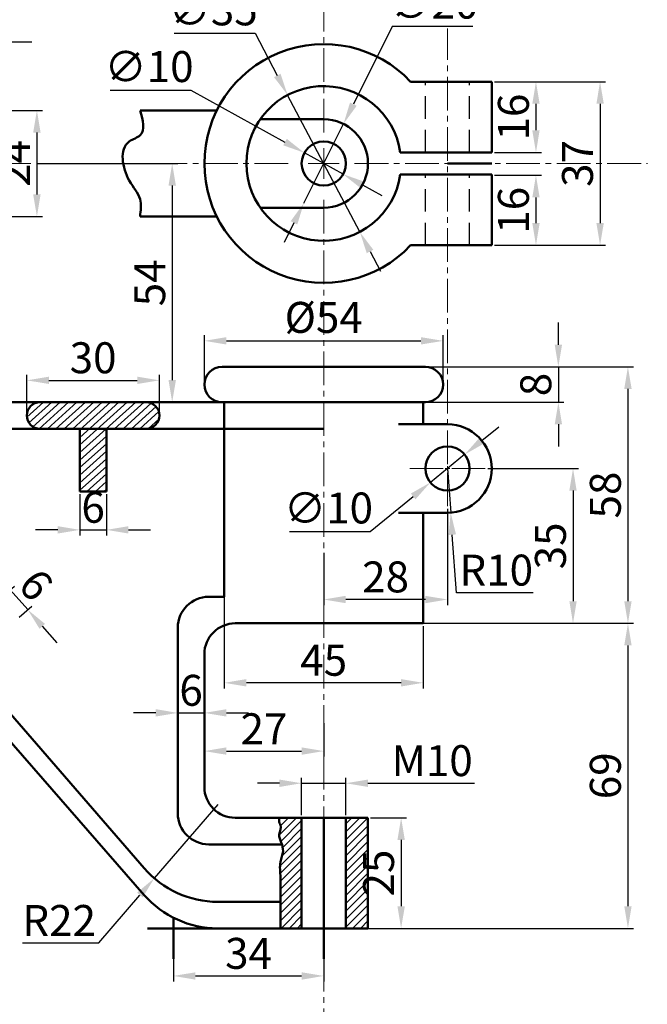
# Model space of a CAD drawing. Units: millimetres. Extents: x 434 to 1535, y -197 to 318.
# Tile 2 of 9: x 579 to 721, y -19 to 204. Entities that reach past the tile are written whole.
import ezdxf

# ---------------------------------------------------------------- set-up
doc = ezdxf.new("R2010")
doc.units = ezdxf.units.MM
doc.header["$LTSCALE"] = 0.4
doc.linetypes.add('CENTER2', pattern=[28.575, 19.05, -3.175, 3.175, -3.175])
doc.linetypes.add('DASHED', pattern=[19.05, 12.7, -6.35])
for name, color, linetype, lineweight in [('M-CNTR', 1, 'CENTER2', 18), ('M-DIMS', 2, 'Continuous', 25), ('M-HATC', 8, 'Continuous', 18), ('M-HIDN', 6, 'DASHED', 25), ('M-OUTL', 7, 'Continuous', 50)]:
    doc.layers.add(name, color=color, linetype=linetype, lineweight=lineweight)
doc.styles.get("Standard").update_dxf_attribs({"font": 'arial.ttf'})
doc.dimstyles.new('ISO-25', dxfattribs={"dimtxt": 7, "dimasz": 5, "dimexe": 1.25, "dimexo": 0.625, "dimtad": 1, "dimtoh": 1, "dimdec": 0, "dimtxsty": 'Standard', "dimcen": 2.5, "dimadec": 0, "dimazin": 0, "dimtfac": 1, "dimtdec": 0, "dimtmove": 0, "dimatfit": 3, "dimfxl": 1, "dimarcsym": 0})

# ---------------------------------------------------------------- blocks, each defined once
blk = doc.blocks.new('*U1')
at = {"layer": 'M-CNTR', "color": 0, "transparency": 16777216}
for p, q in [((0, 7), (0, 38.5)), ((-38.5, 0), (-7, 0)), ((7, 0), (73.2, 0)), ((0, -198.75), (0, -7))]:
    blk.add_line(p, q, dxfattribs=at)
at = {"layer": 'M-CNTR', "color": 0, "linetype": 'Continuous', "transparency": 16777216}
for p, q in [((0, -3.5), (0, 3.5)), ((-3.5, 0), (3.5, 0))]:
    blk.add_line(p, q, dxfattribs=at)
blk = doc.blocks.new('*U2')
at = {"layer": 'M-CNTR', "color": 0, "transparency": 16777216}
for p, q in [((0, 1), (0, 99.51)), ((-8.5, 0), (-1, 0)), ((1, 0), (8.5, 0)), ((0, -8.5), (0, -1))]:
    blk.add_line(p, q, dxfattribs=at)
at = {"layer": 'M-CNTR', "color": 0, "linetype": 'Continuous', "transparency": 16777216}
for p, q in [((-0.5, 0), (0.5, 0)), ((0, -0.5), (0, 0.5))]:
    blk.add_line(p, q, dxfattribs=at)
blk = doc.blocks.new('*U3')
at = {"layer": 'M-CNTR', "color": 0, "transparency": 16777216}
blk.add_line((-45.89, 0), (45.61, 0), dxfattribs=at)
blk = doc.blocks.new('*D12')
at = {"layer": 'Defpoints', "color": 0, "ltscale": 0.4, "transparency": 16777216}
for p in [(571.58, 199.04), (563.58, 188.56), (571.58, 188.56)]:
    blk.add_point(p, dxfattribs=at)
at = {"layer": 'M-DIMS', "color": 0, "lineweight": -2, "ltscale": 0.4, "transparency": 16777216}
for p, q in [((558.58, 199.04), (553.58, 199.04)), ((563.58, 189.19), (563.58, 200.29)), ((563.58, 199.04), (571.58, 199.04)), ((571.58, 189.19), (571.58, 200.29)), ((576.58, 199.04), (581.58, 199.04))]:
    blk.add_line(p, q, dxfattribs=at)
at = {"layer": 'M-DIMS', "color": 0, "ltscale": 0.4, "transparency": 16777216}
for points in [[(558.58, 199.87), (558.58, 198.21), (563.58, 199.04)], [(576.58, 199.87), (576.58, 198.21), (571.58, 199.04)]]:
    blk.add_solid(points, dxfattribs=at)
at = {"layer": 'M-DIMS', "color": 0, "ltscale": 0.4, "transparency": 16777216, "insert": (567.58, 203.24), "char_height": 7, "attachment_point": 5}
blk.add_mtext('8', dxfattribs=at)
blk = doc.blocks.new('*D13')
at = {"layer": 'Defpoints', "color": 0, "ltscale": 0.4, "transparency": 16777216}
for p in [(571.58, 183.56), (571.58, 159.56), (582.71, 159.56)]:
    blk.add_point(p, dxfattribs=at)
at = {"layer": 'M-DIMS', "color": 0, "lineweight": -2, "ltscale": 0.4, "transparency": 16777216}
for p, q in [((572.2, 183.56), (583.96, 183.56)), ((582.71, 178.56), (582.71, 164.56)), ((572.2, 159.56), (583.96, 159.56))]:
    blk.add_line(p, q, dxfattribs=at)
at = {"layer": 'M-DIMS', "color": 0, "ltscale": 0.4, "transparency": 16777216}
for points in [[(581.87, 178.56), (583.54, 178.56), (582.71, 183.56)], [(581.87, 164.56), (583.54, 164.56), (582.71, 159.56)]]:
    blk.add_solid(points, dxfattribs=at)
at = {"layer": 'M-DIMS', "color": 0, "ltscale": 0.4, "transparency": 16777216, "insert": (578.57, 171.56), "char_height": 7, "attachment_point": 5, "rotation": 90}
blk.add_mtext('24', dxfattribs=at)
blk = doc.blocks.new('*D17')
at = {"layer": 'Defpoints', "color": 0, "ltscale": 0.4, "transparency": 16777216}
for p in [(610.41, 122.51), (580.43, 114.31), (610.41, 114.31)]:
    blk.add_point(p, dxfattribs=at)
at = {"layer": 'M-DIMS', "color": 0, "lineweight": -2, "ltscale": 0.4, "transparency": 16777216}
for p, q in [((580.43, 114.93), (580.43, 123.76)), ((585.43, 122.51), (605.41, 122.51)), ((610.41, 114.93), (610.41, 123.76))]:
    blk.add_line(p, q, dxfattribs=at)
at = {"layer": 'M-DIMS', "color": 0, "ltscale": 0.4, "transparency": 16777216}
for points in [[(585.43, 123.34), (585.43, 121.68), (580.43, 122.51)], [(605.41, 123.34), (605.41, 121.68), (610.41, 122.51)]]:
    blk.add_solid(points, dxfattribs=at)
at = {"layer": 'M-DIMS', "color": 0, "ltscale": 0.4, "transparency": 16777216, "insert": (595.42, 126.71), "char_height": 7, "attachment_point": 5}
blk.add_mtext('30', dxfattribs=at)
blk = doc.blocks.new('*D18')
at = {"layer": 'Defpoints', "color": 0, "ltscale": 0.4, "transparency": 16777216}
for p in [(592.42, 97.38), (598.42, 97.38), (598.42, 88.69)]:
    blk.add_point(p, dxfattribs=at)
at = {"layer": 'M-DIMS', "color": 0, "lineweight": -2, "ltscale": 0.4, "transparency": 16777216}
for p, q in [((592.42, 96.75), (592.42, 87.44)), ((598.42, 96.75), (598.42, 87.44)), ((587.42, 88.69), (582.42, 88.69)), ((592.42, 88.69), (598.42, 88.69)), ((603.42, 88.69), (608.42, 88.69))]:
    blk.add_line(p, q, dxfattribs=at)
at = {"layer": 'M-DIMS', "color": 0, "ltscale": 0.4, "transparency": 16777216}
for points in [[(587.42, 89.52), (587.42, 87.86), (592.42, 88.69)], [(603.42, 89.52), (603.42, 87.86), (598.42, 88.69)]]:
    blk.add_solid(points, dxfattribs=at)
at = {"layer": 'M-DIMS', "color": 0, "ltscale": 0.4, "transparency": 16777216, "insert": (595.42, 92.89), "char_height": 7, "attachment_point": 5}
blk.add_mtext('6', dxfattribs=at)
blk = doc.blocks.new('*D19')
at = {"layer": 'Defpoints', "color": 0, "ltscale": 0.4, "transparency": 16777216}
for p in [(613.58, -1.44), (647.58, -2.82), (647.58, -12.21)]:
    blk.add_point(p, dxfattribs=at)
at = {"layer": 'M-DIMS', "color": 0, "lineweight": -2, "ltscale": 0.4, "transparency": 16777216}
for p, q in [((613.58, -2.06), (613.58, -13.46)), ((647.58, -3.45), (647.58, -13.46)), ((618.58, -12.21), (642.58, -12.21))]:
    blk.add_line(p, q, dxfattribs=at)
at = {"layer": 'M-DIMS', "color": 0, "ltscale": 0.4, "transparency": 16777216}
for points in [[(618.58, -11.38), (618.58, -13.05), (613.58, -12.21)], [(642.58, -11.38), (642.58, -13.05), (647.58, -12.21)]]:
    blk.add_solid(points, dxfattribs=at)
at = {"layer": 'M-DIMS', "color": 0, "ltscale": 0.4, "transparency": 16777216, "insert": (630.58, -8.01), "char_height": 7, "attachment_point": 5}
blk.add_mtext('34', dxfattribs=at)
blk = doc.blocks.new('*D21')
at = {"layer": 'Defpoints', "color": 0, "ltscale": 0.4, "transparency": 16777216}
for p in [(574.27, 73.05), (580.63, 70.64), (578.22, 68.53)]:
    blk.add_point(p, dxfattribs=at)
at = {"layer": 'M-DIMS', "color": 0, "lineweight": -2, "ltscale": 0.4, "transparency": 16777216}
for p, q in [((573.4, 78.92), (570.11, 82.68)), ((574.74, 73.46), (577.63, 75.98)), ((576.69, 75.15), (580.63, 70.64)), ((578.69, 68.94), (581.58, 71.46)), ((583.92, 66.87), (587.21, 63.11))]:
    blk.add_line(p, q, dxfattribs=at)
at = {"layer": 'M-DIMS', "color": 0, "ltscale": 0.4, "transparency": 16777216}
for points in [[(574.02, 79.47), (572.77, 78.37), (576.69, 75.15)], [(584.55, 67.42), (583.3, 66.32), (580.63, 70.64)]]:
    blk.add_solid(points, dxfattribs=at)
at = {"layer": 'M-DIMS', "color": 0, "ltscale": 0.4, "transparency": 16777216, "insert": (581.82, 75.66), "char_height": 7, "attachment_point": 5, "rotation": 311.1518}
blk.add_mtext('6', dxfattribs=at)
blk = doc.blocks.new('*D22')
at = {"layer": 'Defpoints', "color": 0, "ltscale": 0.4, "transparency": 16777216}
for p in [(582.08, 171.56), (580.43, 117.56), (613.31, 117.56)]:
    blk.add_point(p, dxfattribs=at)
at = {"layer": 'M-DIMS', "color": 0, "lineweight": -2, "ltscale": 0.4, "transparency": 16777216}
for p, q in [((582.71, 171.56), (614.56, 171.56)), ((613.31, 166.56), (613.31, 122.56)), ((581.05, 117.56), (614.56, 117.56))]:
    blk.add_line(p, q, dxfattribs=at)
at = {"layer": 'M-DIMS', "color": 0, "ltscale": 0.4, "transparency": 16777216}
for points in [[(612.48, 166.56), (614.15, 166.56), (613.31, 171.56)], [(612.48, 122.56), (614.15, 122.56), (613.31, 117.56)]]:
    blk.add_solid(points, dxfattribs=at)
at = {"layer": 'M-DIMS', "color": 0, "ltscale": 0.4, "transparency": 16777216, "insert": (609.13, 144.56), "char_height": 7, "attachment_point": 5, "rotation": 90}
blk.add_mtext('54', dxfattribs=at)
blk = doc.blocks.new('*D23')
at = {"layer": 'Defpoints', "color": 0, "ltscale": 0.4, "transparency": 16777216}
for p in [(674.58, 131.44), (620.58, 121.56), (674.58, 121.56)]:
    blk.add_point(p, dxfattribs=at)
at = {"layer": 'M-DIMS', "color": 0, "lineweight": -2, "ltscale": 0.4, "transparency": 16777216}
for p, q in [((620.58, 122.19), (620.58, 132.69)), ((625.58, 131.44), (669.58, 131.44)), ((674.58, 122.19), (674.58, 132.69))]:
    blk.add_line(p, q, dxfattribs=at)
at = {"layer": 'M-DIMS', "color": 0, "ltscale": 0.4, "transparency": 16777216}
for points in [[(625.58, 132.28), (625.58, 130.61), (620.58, 131.44)], [(669.58, 132.28), (669.58, 130.61), (674.58, 131.44)]]:
    blk.add_solid(points, dxfattribs=at)
at = {"layer": 'M-DIMS', "color": 0, "ltscale": 0.4, "transparency": 16777216, "insert": (647.58, 135.84), "char_height": 7, "attachment_point": 5}
blk.add_mtext('%%C54', dxfattribs=at)
blk = doc.blocks.new('*D24')
at = {"layer": 'Defpoints', "color": 0, "ltscale": 0.4, "transparency": 16777216}
for p in [(685.58, 190.06), (685.58, 174.06), (695.59, 174.06)]:
    blk.add_point(p, dxfattribs=at)
at = {"layer": 'M-DIMS', "color": 0, "lineweight": -2, "ltscale": 0.4, "transparency": 16777216}
for p, q in [((686.2, 190.06), (696.84, 190.06)), ((695.59, 185.06), (695.59, 179.06)), ((686.2, 174.06), (696.84, 174.06))]:
    blk.add_line(p, q, dxfattribs=at)
at = {"layer": 'M-DIMS', "color": 0, "ltscale": 0.4, "transparency": 16777216}
for points in [[(694.76, 185.06), (696.42, 185.06), (695.59, 190.06)], [(694.76, 179.06), (696.42, 179.06), (695.59, 174.06)]]:
    blk.add_solid(points, dxfattribs=at)
at = {"layer": 'M-DIMS', "color": 0, "ltscale": 0.4, "transparency": 16777216, "insert": (691.39, 182.06), "char_height": 7, "attachment_point": 5, "rotation": 90}
blk.add_mtext('16', dxfattribs=at)
blk = doc.blocks.new('*D25')
at = {"layer": 'Defpoints', "color": 0, "ltscale": 0.4, "transparency": 16777216}
for p in [(685.58, 168.88), (685.58, 153.06), (695.59, 153.06)]:
    blk.add_point(p, dxfattribs=at)
at = {"layer": 'M-DIMS', "color": 0, "lineweight": -2, "ltscale": 0.4, "transparency": 16777216}
for p, q in [((686.2, 168.88), (696.84, 168.88)), ((695.59, 163.88), (695.59, 158.06)), ((686.2, 153.06), (696.84, 153.06))]:
    blk.add_line(p, q, dxfattribs=at)
at = {"layer": 'M-DIMS', "color": 0, "ltscale": 0.4, "transparency": 16777216}
for points in [[(694.76, 163.88), (696.42, 163.88), (695.59, 168.88)], [(694.76, 158.06), (696.42, 158.06), (695.59, 153.06)]]:
    blk.add_solid(points, dxfattribs=at)
at = {"layer": 'M-DIMS', "color": 0, "ltscale": 0.4, "transparency": 16777216, "insert": (691.39, 160.97), "char_height": 7, "attachment_point": 5, "rotation": 90}
blk.add_mtext('16', dxfattribs=at)
blk = doc.blocks.new('*D26')
at = {"layer": 'Defpoints', "color": 0, "ltscale": 0.4, "transparency": 16777216}
for p in [(670.58, 125.56), (670.08, 117.56), (700.66, 117.56)]:
    blk.add_point(p, dxfattribs=at)
at = {"layer": 'M-DIMS', "color": 0, "lineweight": -2, "ltscale": 0.4, "transparency": 16777216}
for p, q in [((700.66, 130.56), (700.66, 135.56)), ((671.2, 125.56), (701.91, 125.56)), ((700.66, 125.56), (700.66, 117.56)), ((670.7, 117.56), (701.91, 117.56)), ((700.66, 112.56), (700.66, 107.56))]:
    blk.add_line(p, q, dxfattribs=at)
at = {"layer": 'M-DIMS', "color": 0, "ltscale": 0.4, "transparency": 16777216}
for points in [[(699.83, 130.56), (701.49, 130.56), (700.66, 125.56)], [(699.83, 112.56), (701.49, 112.56), (700.66, 117.56)]]:
    blk.add_solid(points, dxfattribs=at)
at = {"layer": 'M-DIMS', "color": 0, "ltscale": 0.4, "transparency": 16777216, "insert": (696.46, 121.56), "char_height": 7, "attachment_point": 5, "rotation": 90}
blk.add_mtext('8', dxfattribs=at)
blk = doc.blocks.new('*D27')
at = {"layer": 'Defpoints', "color": 0, "ltscale": 0.4, "transparency": 16777216}
for p in [(690.31, 125.56), (660.09, 67.56), (716.39, 67.56)]:
    blk.add_point(p, dxfattribs=at)
at = {"layer": 'M-DIMS', "color": 0, "lineweight": -2, "ltscale": 0.4, "transparency": 16777216}
for p, q in [((690.93, 125.56), (717.64, 125.56)), ((716.39, 120.56), (716.39, 72.56)), ((660.71, 67.56), (717.64, 67.56))]:
    blk.add_line(p, q, dxfattribs=at)
at = {"layer": 'M-DIMS', "color": 0, "ltscale": 0.4, "transparency": 16777216}
for points in [[(715.56, 120.56), (717.23, 120.56), (716.39, 125.56)], [(715.56, 72.56), (717.23, 72.56), (716.39, 67.56)]]:
    blk.add_solid(points, dxfattribs=at)
at = {"layer": 'M-DIMS', "color": 0, "ltscale": 0.4, "transparency": 16777216, "insert": (712.19, 96.56), "char_height": 7, "attachment_point": 5, "rotation": 90}
blk.add_mtext('58', dxfattribs=at)
blk = doc.blocks.new('*D28')
at = {"layer": 'Defpoints', "color": 0, "ltscale": 0.4, "transparency": 16777216}
for p in [(657.58, 23.56), (657.58, -1.44), (665.09, -1.44)]:
    blk.add_point(p, dxfattribs=at)
at = {"layer": 'M-DIMS', "color": 0, "lineweight": -2, "ltscale": 0.4, "transparency": 16777216}
for p, q in [((658.2, 23.56), (666.34, 23.56)), ((665.09, 18.56), (665.09, 3.56)), ((658.2, -1.44), (666.34, -1.44))]:
    blk.add_line(p, q, dxfattribs=at)
at = {"layer": 'M-DIMS', "color": 0, "ltscale": 0.4, "transparency": 16777216}
for points in [[(664.26, 18.56), (665.93, 18.56), (665.09, 23.56)], [(664.26, 3.56), (665.93, 3.56), (665.09, -1.44)]]:
    blk.add_solid(points, dxfattribs=at)
at = {"layer": 'M-DIMS', "color": 0, "ltscale": 0.4, "transparency": 16777216, "insert": (660.89, 11.06), "char_height": 7, "attachment_point": 5, "rotation": 90}
blk.add_mtext('25', dxfattribs=at)
blk = doc.blocks.new('*D29')
at = {"layer": 'Defpoints', "color": 0, "ltscale": 0.4, "transparency": 16777216}
for p in [(652.58, 31.38), (642.58, 23.56), (652.58, 23.56)]:
    blk.add_point(p, dxfattribs=at)
at = {"layer": 'M-DIMS', "color": 0, "lineweight": -2, "ltscale": 0.4, "transparency": 16777216}
for p, q in [((637.58, 31.38), (632.58, 31.38)), ((642.58, 24.19), (642.58, 32.63)), ((642.58, 31.38), (652.58, 31.38)), ((652.58, 24.19), (652.58, 32.63)), ((657.58, 31.38), (681.65, 31.38))]:
    blk.add_line(p, q, dxfattribs=at)
at = {"layer": 'M-DIMS', "color": 0, "ltscale": 0.4, "transparency": 16777216}
for points in [[(637.58, 32.21), (637.58, 30.54), (642.58, 31.38)], [(657.58, 32.21), (657.58, 30.54), (652.58, 31.38)]]:
    blk.add_solid(points, dxfattribs=at)
at = {"layer": 'M-DIMS', "color": 0, "ltscale": 0.4, "transparency": 16777216, "insert": (672.11, 35.58), "char_height": 7, "attachment_point": 5}
blk.add_mtext('M10', dxfattribs=at)
blk = doc.blocks.new('*D30')
at = {"layer": 'Defpoints', "color": 0, "ltscale": 0.4, "transparency": 16777216}
for p in [(614.58, 52.82), (620.58, 52.82), (620.58, 47.29)]:
    blk.add_point(p, dxfattribs=at)
at = {"layer": 'M-DIMS', "color": 0, "lineweight": -2, "ltscale": 0.4, "transparency": 16777216}
for p, q in [((614.58, 52.2), (614.58, 46.04)), ((620.58, 52.2), (620.58, 46.04)), ((609.58, 47.29), (604.58, 47.29)), ((614.58, 47.29), (620.58, 47.29)), ((625.58, 47.29), (630.58, 47.29))]:
    blk.add_line(p, q, dxfattribs=at)
at = {"layer": 'M-DIMS', "color": 0, "ltscale": 0.4, "transparency": 16777216}
for points in [[(609.58, 48.13), (609.58, 46.46), (614.58, 47.29)], [(625.58, 48.13), (625.58, 46.46), (620.58, 47.29)]]:
    blk.add_solid(points, dxfattribs=at)
at = {"layer": 'M-DIMS', "color": 0, "ltscale": 0.4, "transparency": 16777216, "insert": (617.58, 51.49), "char_height": 7, "attachment_point": 5}
blk.add_mtext('6', dxfattribs=at)
blk = doc.blocks.new('*D31')
at = {"layer": 'Defpoints', "color": 0, "ltscale": 0.4, "transparency": 16777216}
for p in [(620.58, 45.56), (647.58, 45.56), (647.58, 38.65)]:
    blk.add_point(p, dxfattribs=at)
at = {"layer": 'M-DIMS', "color": 0, "lineweight": -2, "ltscale": 0.4, "transparency": 16777216}
for p, q in [((620.58, 44.94), (620.58, 37.4)), ((647.58, 44.94), (647.58, 37.4)), ((625.58, 38.65), (642.58, 38.65))]:
    blk.add_line(p, q, dxfattribs=at)
at = {"layer": 'M-DIMS', "color": 0, "ltscale": 0.4, "transparency": 16777216}
for points in [[(625.58, 39.49), (625.58, 37.82), (620.58, 38.65)], [(642.58, 39.49), (642.58, 37.82), (647.58, 38.65)]]:
    blk.add_solid(points, dxfattribs=at)
at = {"layer": 'M-DIMS', "color": 0, "ltscale": 0.4, "transparency": 16777216, "insert": (634.08, 42.79), "char_height": 7, "attachment_point": 5}
blk.add_mtext('27', dxfattribs=at)
blk = doc.blocks.new('*D32')
at = {"layer": 'Defpoints', "color": 0, "ltscale": 0.4, "transparency": 16777216}
for p in [(623.62, 26.56), (609.26, 9.89)]:
    blk.add_point(p, dxfattribs=at)
at = {"layer": 'M-DIMS', "color": 0, "lineweight": -2, "ltscale": 0.4, "transparency": 16777216}
for p, q in [((623.62, 26.56), (609.26, 9.89)), ((596.7, -4.71), (606, 6.1)), ((579.42, -4.71), (596.7, -4.71))]:
    blk.add_line(p, q, dxfattribs=at)
at = {"layer": 'M-DIMS', "color": 0, "ltscale": 0.4, "transparency": 16777216}
blk.add_solid([(605.37, 6.64), (606.63, 5.55), (609.26, 9.89)], dxfattribs=at)
at = {"layer": 'M-DIMS', "color": 0, "ltscale": 0.4, "transparency": 16777216, "insert": (587.74, -0.57), "char_height": 7, "attachment_point": 5}
blk.add_mtext('R22', dxfattribs=at)
blk = doc.blocks.new('*D33')
at = {"layer": 'Defpoints', "color": 0, "ltscale": 0.4, "transparency": 16777216}
for p in [(675.58, 102.56), (676.3, 92.59)]:
    blk.add_point(p, dxfattribs=at)
at = {"layer": 'M-DIMS', "color": 0, "lineweight": -2, "ltscale": 0.4, "transparency": 16777216}
for p, q in [((675.58, 102.56), (676.3, 92.59)), ((677.63, 74.48), (676.67, 87.6)), ((694.95, 74.48), (677.63, 74.48))]:
    blk.add_line(p, q, dxfattribs=at)
at = {"layer": 'M-DIMS', "color": 0, "ltscale": 0.4, "transparency": 16777216}
blk.add_solid([(677.5, 87.66), (675.84, 87.54), (676.3, 92.59)], dxfattribs=at)
at = {"layer": 'M-DIMS', "color": 0, "ltscale": 0.4, "transparency": 16777216, "insert": (686.6, 78.68), "char_height": 7, "attachment_point": 5}
blk.add_mtext('R10', dxfattribs=at)
blk = doc.blocks.new('*D34')
at = {"layer": 'Defpoints', "color": 0, "ltscale": 0.4, "transparency": 16777216}
for p in [(679.45, 105.72), (671.7, 99.41)]:
    blk.add_point(p, dxfattribs=at)
at = {"layer": 'M-DIMS', "color": 0, "lineweight": -2, "ltscale": 0.4, "transparency": 16777216}
for p, q in [((683.33, 108.87), (687.21, 112.03)), ((679.45, 105.72), (671.7, 99.41)), ((658.09, 88.34), (667.82, 96.25)), ((639.85, 88.34), (658.09, 88.34))]:
    blk.add_line(p, q, dxfattribs=at)
at = {"layer": 'M-DIMS', "color": 0, "ltscale": 0.4, "transparency": 16777216}
for points in [[(682.81, 109.52), (683.86, 108.23), (679.45, 105.72)], [(667.29, 96.9), (668.34, 95.6), (671.7, 99.41)]]:
    blk.add_solid(points, dxfattribs=at)
at = {"layer": 'M-DIMS', "color": 0, "ltscale": 0.4, "transparency": 16777216, "insert": (648.66, 92.73), "char_height": 7, "attachment_point": 5}
blk.add_mtext('∅10', dxfattribs=at)
blk = doc.blocks.new('*D35')
at = {"layer": 'Defpoints', "color": 0, "ltscale": 0.4, "transparency": 16777216}
for p in [(684.08, 102.56), (684.08, 67.56), (703.97, 67.56)]:
    blk.add_point(p, dxfattribs=at)
at = {"layer": 'M-DIMS', "color": 0, "lineweight": -2, "ltscale": 0.4, "transparency": 16777216}
for p, q in [((684.7, 102.56), (705.22, 102.56)), ((703.97, 97.56), (703.97, 72.56)), ((684.7, 67.56), (705.22, 67.56))]:
    blk.add_line(p, q, dxfattribs=at)
at = {"layer": 'M-DIMS', "color": 0, "ltscale": 0.4, "transparency": 16777216}
for points in [[(703.14, 97.56), (704.8, 97.56), (703.97, 102.56)], [(703.14, 72.56), (704.8, 72.56), (703.97, 67.56)]]:
    blk.add_solid(points, dxfattribs=at)
at = {"layer": 'M-DIMS', "color": 0, "ltscale": 0.4, "transparency": 16777216, "insert": (699.77, 85.06), "char_height": 7, "attachment_point": 5, "rotation": 90}
blk.add_mtext('35', dxfattribs=at)
blk = doc.blocks.new('*D36')
at = {"layer": 'Defpoints', "color": 0, "ltscale": 0.4, "transparency": 16777216}
for p in [(685.58, 190.06), (685.58, 153.06), (710.09, 153.06)]:
    blk.add_point(p, dxfattribs=at)
at = {"layer": 'M-DIMS', "color": 0, "lineweight": -2, "ltscale": 0.4, "transparency": 16777216}
for p, q in [((686.2, 190.06), (711.34, 190.06)), ((710.09, 185.06), (710.09, 158.06)), ((686.2, 153.06), (711.34, 153.06))]:
    blk.add_line(p, q, dxfattribs=at)
at = {"layer": 'M-DIMS', "color": 0, "ltscale": 0.4, "transparency": 16777216}
for points in [[(709.26, 185.06), (710.93, 185.06), (710.09, 190.06)], [(709.26, 158.06), (710.93, 158.06), (710.09, 153.06)]]:
    blk.add_solid(points, dxfattribs=at)
at = {"layer": 'M-DIMS', "color": 0, "ltscale": 0.4, "transparency": 16777216, "insert": (705.89, 171.56), "char_height": 7, "attachment_point": 5, "rotation": 90}
blk.add_mtext('37', dxfattribs=at)
blk = doc.blocks.new('*D37')
at = {"layer": 'Defpoints', "color": 0, "ltscale": 0.4, "transparency": 16777216}
for p in [(670.08, 67.56), (647.58, -1.44), (716.39, -1.44)]:
    blk.add_point(p, dxfattribs=at)
at = {"layer": 'M-DIMS', "color": 0, "lineweight": -2, "ltscale": 0.4, "transparency": 16777216}
for p, q in [((670.7, 67.56), (717.64, 67.56)), ((716.39, 62.56), (716.39, 3.56)), ((648.2, -1.44), (717.64, -1.44))]:
    blk.add_line(p, q, dxfattribs=at)
at = {"layer": 'M-DIMS', "color": 0, "ltscale": 0.4, "transparency": 16777216}
for points in [[(715.56, 62.56), (717.23, 62.56), (716.39, 67.56)], [(715.56, 3.56), (717.23, 3.56), (716.39, -1.44)]]:
    blk.add_solid(points, dxfattribs=at)
at = {"layer": 'M-DIMS', "color": 0, "ltscale": 0.4, "transparency": 16777216, "insert": (712.19, 33.06), "char_height": 7, "attachment_point": 5, "rotation": 90}
blk.add_mtext('69', dxfattribs=at)
blk = doc.blocks.new('*D38')
at = {"layer": 'Defpoints', "color": 0, "ltscale": 0.4, "transparency": 16777216}
for p in [(625.08, 80.85), (670.08, 67.56), (625.08, 54.09)]:
    blk.add_point(p, dxfattribs=at)
at = {"layer": 'M-DIMS', "color": 0, "lineweight": -2, "ltscale": 0.4, "transparency": 16777216}
for p, q in [((625.08, 80.23), (625.08, 52.84)), ((670.08, 66.94), (670.08, 52.84)), ((665.08, 54.09), (630.08, 54.09))]:
    blk.add_line(p, q, dxfattribs=at)
at = {"layer": 'M-DIMS', "color": 0, "ltscale": 0.4, "transparency": 16777216}
for points in [[(630.08, 54.93), (630.08, 53.26), (625.08, 54.09)], [(665.08, 54.93), (665.08, 53.26), (670.08, 54.09)]]:
    blk.add_solid(points, dxfattribs=at)
at = {"layer": 'M-DIMS', "color": 0, "ltscale": 0.4, "transparency": 16777216, "insert": (647.58, 58.28), "char_height": 7, "attachment_point": 5}
blk.add_mtext('45', dxfattribs=at)
blk = doc.blocks.new('*D39')
at = {"layer": 'Defpoints', "color": 0, "ltscale": 0.4, "transparency": 16777216}
for p in [(675.58, 94.06), (647.58, 84.11), (647.58, 72.94)]:
    blk.add_point(p, dxfattribs=at)
at = {"layer": 'M-DIMS', "color": 0, "lineweight": -2, "ltscale": 0.4, "transparency": 16777216}
for p, q in [((675.58, 93.44), (675.58, 71.69)), ((647.58, 83.49), (647.58, 71.69)), ((670.58, 72.94), (652.58, 72.94))]:
    blk.add_line(p, q, dxfattribs=at)
at = {"layer": 'M-DIMS', "color": 0, "ltscale": 0.4, "transparency": 16777216}
for points in [[(652.58, 73.77), (652.58, 72.1), (647.58, 72.94)], [(670.58, 73.77), (670.58, 72.1), (675.58, 72.94)]]:
    blk.add_solid(points, dxfattribs=at)
at = {"layer": 'M-DIMS', "color": 0, "ltscale": 0.4, "transparency": 16777216, "insert": (661.58, 77.14), "char_height": 7, "attachment_point": 5}
blk.add_mtext('28', dxfattribs=at)
blk = doc.blocks.new('*D40')
at = {"layer": 'Defpoints', "color": 0, "ltscale": 0.4, "transparency": 16777216}
for p in [(639.42, 187.04), (655.74, 156.08)]:
    blk.add_point(p, dxfattribs=at)
at = {"layer": 'M-DIMS', "color": 0, "lineweight": -2, "ltscale": 0.4, "transparency": 16777216}
for p, q in [((613.74, 201), (632.06, 201)), ((632.06, 201), (637.08, 191.46)), ((655.74, 156.08), (639.42, 187.04)), ((658.07, 151.66), (660.4, 147.23))]:
    blk.add_line(p, q, dxfattribs=at)
at = {"layer": 'M-DIMS', "color": 0, "ltscale": 0.4, "transparency": 16777216}
for points in [[(637.82, 191.85), (636.35, 191.08), (639.42, 187.04)], [(658.8, 152.04), (657.33, 151.27), (655.74, 156.08)]]:
    blk.add_solid(points, dxfattribs=at)
at = {"layer": 'M-DIMS', "color": 0, "ltscale": 0.4, "transparency": 16777216, "insert": (622.58, 205.4), "char_height": 7, "attachment_point": 5}
blk.add_mtext('∅35', dxfattribs=at)
blk = doc.blocks.new('*D41')
at = {"layer": 'Defpoints', "color": 0, "ltscale": 0.4, "transparency": 16777216}
for p in [(652.05, 180.5), (643.1, 162.62)]:
    blk.add_point(p, dxfattribs=at)
at = {"layer": 'M-DIMS', "color": 0, "lineweight": -2, "ltscale": 0.4, "transparency": 16777216}
for p, q in [((663.07, 202.52), (654.29, 184.97)), ((681.32, 202.52), (663.07, 202.52)), ((643.1, 162.62), (652.05, 180.5)), ((640.86, 158.15), (638.62, 153.68))]:
    blk.add_line(p, q, dxfattribs=at)
at = {"layer": 'M-DIMS', "color": 0, "ltscale": 0.4, "transparency": 16777216}
for points in [[(653.54, 185.35), (655.03, 184.6), (652.05, 180.5)], [(640.12, 158.52), (641.61, 157.77), (643.1, 162.62)]]:
    blk.add_solid(points, dxfattribs=at)
at = {"layer": 'M-DIMS', "color": 0, "ltscale": 0.4, "transparency": 16777216, "insert": (672.51, 206.92), "char_height": 7, "attachment_point": 5}
blk.add_mtext('∅20', dxfattribs=at)
blk = doc.blocks.new('*D42')
at = {"layer": 'Defpoints', "color": 0, "ltscale": 0.4, "transparency": 16777216}
for p in [(643.2, 173.98), (651.95, 169.14)]:
    blk.add_point(p, dxfattribs=at)
at = {"layer": 'M-DIMS', "color": 0, "lineweight": -2, "ltscale": 0.4, "transparency": 16777216}
for p, q in [((599.27, 188.17), (617.52, 188.17)), ((617.52, 188.17), (638.82, 176.4)), ((651.95, 169.14), (643.2, 173.98)), ((656.33, 166.72), (660.7, 164.31))]:
    blk.add_line(p, q, dxfattribs=at)
at = {"layer": 'M-DIMS', "color": 0, "ltscale": 0.4, "transparency": 16777216}
for points in [[(639.23, 177.13), (638.42, 175.67), (643.2, 173.98)], [(656.73, 167.45), (655.92, 165.99), (651.95, 169.14)]]:
    blk.add_solid(points, dxfattribs=at)
at = {"layer": 'M-DIMS', "color": 0, "ltscale": 0.4, "transparency": 16777216, "insert": (608.08, 192.57), "char_height": 7, "attachment_point": 5}
blk.add_mtext('∅10', dxfattribs=at)

msp = doc.modelspace()

# ---------------------------------------------------------------- hatches: boundary and pattern name
at = {"layer": 'M-HATC', "ltscale": 0.4}
h = msp.add_hatch(dxfattribs=at)
h.set_pattern_fill('ANSI31', color=256, scale=0.4, angle=177)
h.paths.add_polyline_path([(607.42, 117.56), (583.42, 117.56, 1), (583.42, 111.56), (607.42, 111.56, 1)])
h.paths.add_polyline_path([(598.42, 111.56), (592.42, 111.56), (592.42, 97.38), (598.42, 97.38)])
h = msp.add_hatch(dxfattribs=at)
h.set_pattern_fill('ANSI31', color=256, scale=0.4)
h.paths.add_polyline_path([(652.58, -1.44), (657.58, -1.44), (657.58, 23.56), (652.58, 23.56)])
edge = h.paths.add_edge_path()
edge.add_line((642.58, 23.56), (637.58, 23.56))
edge.add_spline(control_points=[(637.58, 23.56), (637.49, 23.14), (637.38, 22.54), (638.26, 21.48), (637.09, 19.84), (638.07, 17.96), (638.63, 15.84), (637.45, 13.27), (637.91, 10.18), (637.78, 6.47), (637.82, 2.64), (637.82, -0.15), (637.82, -1.44)], knot_values=[0, 0, 0, 0, 1.185966, 1.713035, 3.854844, 5.735548, 7.773019, 10.207895, 13.797946, 16.902491, 21.388461, 25.266792, 25.266792, 25.266792, 25.266792], degree=3, periodic=0)
edge.add_line((637.82, -1.44), (642.58, -1.44))
edge.add_line((642.58, -1.44), (642.58, 23.56))

# ---------------------------------------------------------------- linework, layer by layer
at = {"layer": 'M-HIDN'}
for p, q in [((670.58, 174.06), (670.58, 190.06)), ((680.58, 174.06), (680.58, 190.06)), ((670.58, 153.06), (670.58, 169.06)), ((680.58, 153.06), (680.58, 169.06))]:
    msp.add_line(p, q, dxfattribs=at)
at = {"layer": 'M-OUTL'}
for p, q in [((667.24, 190.06), (685.58, 190.06)), ((685.58, 174.06), (685.58, 190.06)), ((664.9, 174.06), (685.58, 174.06)), ((675.58, 171.56), (685.58, 171.56)), ((664.9, 169.06), (685.58, 169.06)), ((685.58, 153.06), (685.58, 169.06)), ((667.24, 153.06), (685.58, 153.06)), ((625.08, 73.56), (625.08, 117.56)), ((670.08, 112.56), (670.08, 117.56)), ((675.58, 112.56), (664.53, 112.56)), ((675.58, 92.56), (664.46, 92.56)), ((670.08, 67.56), (670.08, 92.56)), ((625.08, 73.56), (621.58, 73.56)), ((670.08, 67.56), (627.58, 67.56)), ((647.58, 67.56), (627.58, 67.56)), ((627.58, 23.56), (657.58, 23.56)), ((623.57, -1.44), (657.58, -1.44))]:
    msp.add_line(p, q, dxfattribs=at)
at = {"layer": 'M-OUTL', "ltscale": 0.4}
for p, q in [((606.09, 183.56), (623.39, 183.56)), ((647.58, 181.56), (633.21, 181.56)), ((647.58, 161.56), (633.21, 161.56)), ((606.04, 159.56), (623.39, 159.56)), ((647.58, 117.56), (575.58, 117.56)), ((647.58, 111.56), (569.58, 111.56)), ((592.42, 111.56), (592.42, 97.38)), ((598.42, 111.56), (598.42, 97.38)), ((516.24, 109.93), (607, 6.08)), ((607, 12.15), (522.18, 109.95)), ((592.42, 97.38), (598.42, 97.38)), ((614.58, 66.56), (614.58, 24.56)), ((620.58, 60.56), (620.58, 30.56)), ((642.58, 23.56), (642.58, -1.44)), ((647.58, 23.56), (647.58, -1.44)), ((652.58, 23.56), (652.58, -1.44)), ((657.58, 23.56), (657.58, -1.44)), ((621.58, 17.56), (638.13, 17.56)), ((623.62, 4.56), (637.81, 4.56)), ((613.58, 0.95), (613.58, -8.33)), ((623.57, -1.44), (607.73, -1.44)), ((647.58, -1.44), (647.58, -8.33))]:
    msp.add_line(p, q, dxfattribs=at)
at = {"layer": 'M-OUTL'}
msp.add_lwpolyline([(624.58, 125.56, 1), (624.58, 117.56), (670.58, 117.56, 1), (670.58, 125.56), (647.58, 125.56)], format="xyb", close=True, dxfattribs=at)
at = {"layer": 'M-OUTL', "ltscale": 0.4}
msp.add_circle((647.58, 171.56), 5, dxfattribs=at)
at = {"layer": 'M-OUTL'}
msp.add_circle((675.58, 102.56), 5, dxfattribs=at)
for centre, radius, start, end in [((647.58, 171.56), 27, 43.2502, 316.7498), ((647.58, 171.56), 17.5, 8.2132, 351.7868), ((675.58, 102.56), 10, 270, 90), ((627.58, 30.56), 7, 180, 270), ((623.57, 20.56), 22, 221.1518, 270)]:
    msp.add_arc(centre, radius, start, end, dxfattribs=at)
at = {"layer": 'M-OUTL', "ltscale": 0.4}
for centre, radius, start, end in [((647.58, 171.56), 10, 270, 90), ((583.42, 114.56), 3, 90, 270), ((607.42, 114.56), 3, 270, 90), ((621.58, 66.56), 7, 90, 180), ((627.58, 60.56), 7, 90, 180), ((621.58, 24.56), 7, 180, 270), ((623.62, 26.56), 22, 220.9337, 270)]:
    msp.add_arc(centre, radius, start, end, dxfattribs=at)
for points, knots in [([(606.09, 183.56), (606.69, 181.33), (607.61, 177.96), (600.99, 176.19), (602.41, 168.24), (606.56, 164.01), (606.2, 160.93), (606.04, 159.56)], [0, 0, 0, 0, 5.592494, 8.464699, 17.29445, 22.169338, 26.089214, 26.089214, 26.089214, 26.089214]), ([(637.58, 23.56), (637.49, 23.14), (637.38, 22.54), (638.26, 21.48), (637.09, 19.84), (638.07, 17.96), (638.63, 15.84), (637.45, 13.27), (637.91, 10.18), (637.78, 6.47), (637.82, 2.64), (637.82, -0.15), (637.82, -1.44)], [0, 0, 0, 0, 1.185966, 1.713035, 3.854844, 5.735548, 7.773019, 10.207895, 13.797946, 16.902491, 21.388461, 25.266792, 25.266792, 25.266792, 25.266792])]:
    msp.add_open_spline(points, degree=3, knots=knots, dxfattribs=at)

# ---------------------------------------------------------------- block references
at = {"layer": 'M-CNTR'}
for name, p in [('*U1', (647.58, 171.56)), ('*U2', (675.58, 102.56)), ('*U3', (539.58, 171.56))]:
    msp.add_blockref(name, p, dxfattribs=at)

# ---------------------------------------------------------------- dimensions: what is measured, and where the dimension line sits
at = {"layer": 'M-DIMS', "ltscale": 0.4}
for p1, p2, picture, middle in [((655.74, 156.08), (639.42, 187.04), '*D40', (622.58, 201)), ((643.1, 162.62), (652.05, 180.5), '*D41', (672.51, 202.52)), ((651.95, 169.14), (643.2, 173.98), '*D42', (608.08, 188.17))]:
    dim = msp.add_diameter_dim_2p(p1=p1, p2=p2, dimstyle='ISO-25', override={"dimclrd": 0, "dimclre": 0, "dimclrt": 0}, dxfattribs=at)
    dim.commit()
    dim.dimension.update_dxf_attribs({"geometry": picture, "text_midpoint": middle, "dimtype": 163})
for base, p1, p2, picture, middle in [((571.58, 199.04), (563.58, 188.56), (571.58, 188.56), '*D12', (567.58, 203.24)), ((610.41, 122.51), (580.43, 114.31), (610.41, 114.31), '*D17', (595.42, 126.71)), ((598.42, 88.69), (592.42, 97.38), (598.42, 97.38), '*D18', (595.42, 92.89)), ((647.58, 72.94), (675.58, 94.06), (647.58, 84.11), '*D39', (661.58, 77.14)), ((647.58, -12.21), (613.58, -1.44), (647.58, -2.82), '*D19', (630.58, -8.01))]:
    dim = msp.add_linear_dim(base=base, p1=p1, p2=p2, dimstyle='ISO-25', override={"dimclrd": 0, "dimclre": 0, "dimclrt": 0}, dxfattribs=at)
    dim.commit()
    dim.dimension.update_dxf_attribs({"geometry": picture, "text_midpoint": middle})
for base, p1, p2, picture, middle in [((695.59, 174.06), (685.58, 190.06), (685.58, 174.06), '*D24', (691.39, 182.06)), ((710.09, 153.06), (685.58, 190.06), (685.58, 153.06), '*D36', (705.89, 171.56)), ((582.71, 159.56), (571.58, 183.56), (571.58, 159.56), '*D13', (578.57, 171.56)), ((613.31, 117.56), (582.08, 171.56), (580.43, 117.56), '*D22', (609.13, 144.56)), ((695.59, 153.06), (685.58, 168.88), (685.58, 153.06), '*D25', (691.39, 160.97)), ((700.66, 117.56), (670.58, 125.56), (670.08, 117.56), '*D26', (696.46, 121.56)), ((716.39, 67.56), (690.31, 125.56), (660.09, 67.56), '*D27', (712.19, 96.56)), ((703.97, 67.56), (684.08, 102.56), (684.08, 67.56), '*D35', (699.77, 85.06)), ((716.39, -1.44), (670.08, 67.56), (647.58, -1.44), '*D37', (712.19, 33.06)), ((665.09, -1.44), (657.58, 23.56), (657.58, -1.44), '*D28', (660.89, 11.06))]:
    dim = msp.add_linear_dim(base=base, p1=p1, p2=p2, angle=90, dimstyle='ISO-25', override={"dimclrd": 0, "dimclre": 0, "dimclrt": 0}, dxfattribs=at)
    dim.commit()
    dim.dimension.update_dxf_attribs({"geometry": picture, "text_midpoint": middle})
for base, p1, p2, text, picture, middle in [((674.58, 131.44), (620.58, 121.56), (674.58, 121.56), '%%C<>', '*D23', (647.58, 135.84)), ((652.58, 31.38), (642.58, 23.56), (652.58, 23.56), 'M<>', '*D29', (672.11, 35.58))]:
    dim = msp.add_linear_dim(base=base, p1=p1, p2=p2, text=text, dimstyle='ISO-25', override={"dimclrd": 0, "dimclre": 0, "dimclrt": 0}, dxfattribs=at)
    dim.commit()
    dim.dimension.update_dxf_attribs({"geometry": picture, "text_midpoint": middle})
dim = msp.add_diameter_dim_2p(p1=(679.45, 105.72), p2=(671.7, 99.41), dimstyle='ISO-25', override={"dimclrd": 0, "dimclre": 0, "dimclrt": 0}, dxfattribs=at)
dim.commit()
dim.dimension.update_dxf_attribs({"geometry": '*D34', "text_midpoint": (648.66, 92.73)})
for center, mpoint, picture, middle in [((675.58, 102.56), (676.3, 92.59), '*D33', (686.6, 74.48)), ((623.62, 26.56), (609.26, 9.89), '*D32', (587.74, -4.71))]:
    dim = msp.add_radius_dim(center=center, mpoint=mpoint, dimstyle='ISO-25', override={"dimclrd": 0, "dimclre": 0, "dimclrt": 0}, dxfattribs=at)
    dim.commit()
    dim.dimension.update_dxf_attribs({"geometry": picture, "text_midpoint": middle, "dimtype": 164})
dim = msp.add_aligned_dim(p1=(574.27, 73.05), p2=(578.22, 68.53), distance=3.2, dimstyle='ISO-25', override={"dimclrd": 0, "dimclre": 0, "dimclrt": 0}, dxfattribs=at)
dim.commit()
dim.dimension.update_dxf_attribs({"geometry": '*D21', "text_midpoint": (581.82, 75.66)})
for base, p1, p2, picture, middle in [((625.08, 54.09), (670.08, 67.56), (625.08, 80.85), '*D38', (647.58, 54.09)), ((620.58, 47.29), (614.58, 52.82), (620.58, 52.82), '*D30', (617.58, 47.29)), ((647.58, 38.65), (620.58, 45.56), (647.58, 45.56), '*D31', (634.08, 38.65))]:
    dim = msp.add_linear_dim(base=base, p1=p1, p2=p2, dimstyle='ISO-25', override={"dimclrd": 0, "dimclre": 0, "dimclrt": 0}, dxfattribs=at)
    dim.commit()
    dim.dimension.update_dxf_attribs({"geometry": picture, "text_midpoint": middle, "dimtype": 160})

doc.saveas('drawing.dxf')
